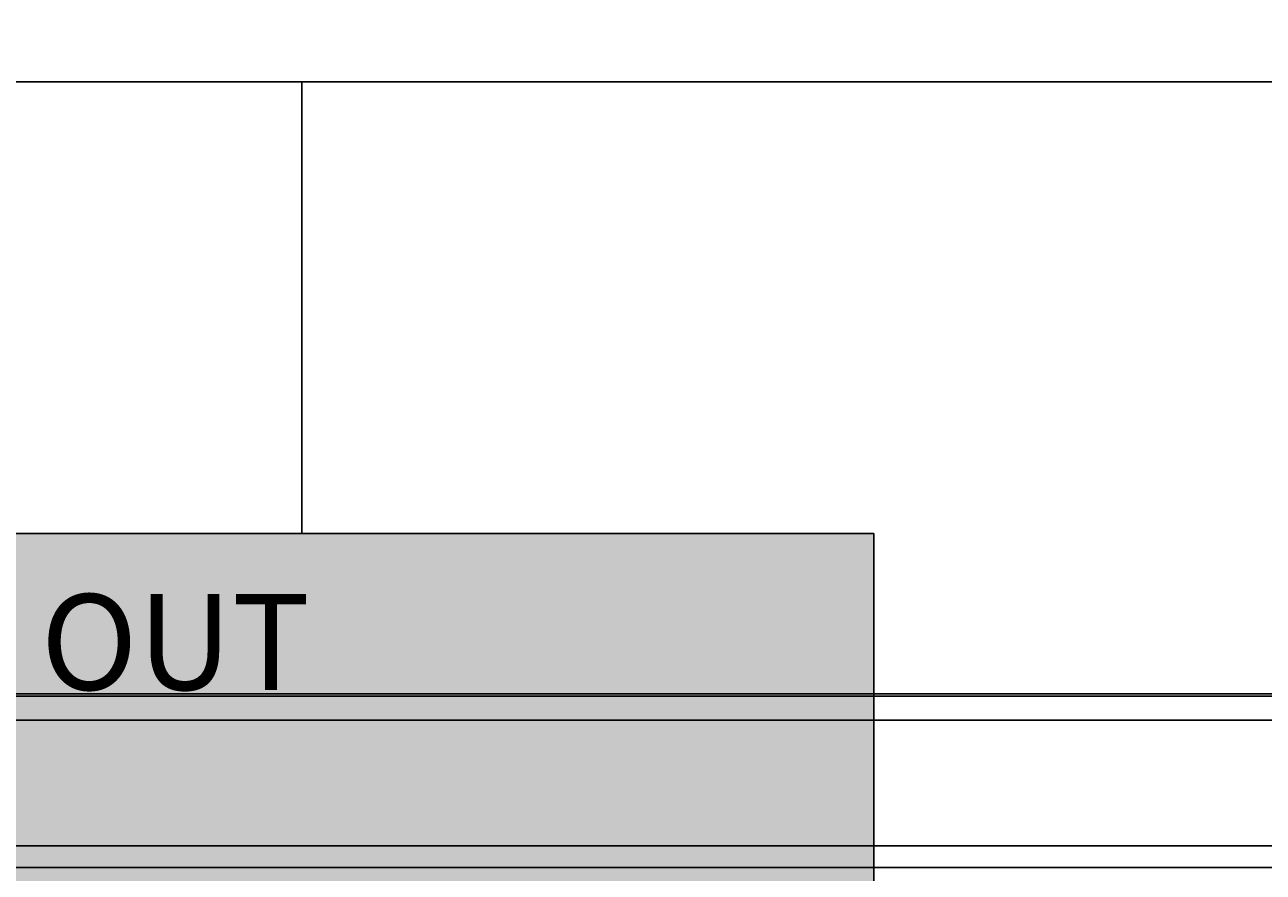
# Model space of a CAD drawing. Units: inches. Extents: x 35362 to 73946, y 43607 to 67532.
# Tile 6 of 134: x 37937 to 40793, y 48909 to 50863. Entities that reach past the tile are written whole.
import ezdxf

# ---------------------------------------------------------------- set-up
doc = ezdxf.new("R2010")
doc.units = ezdxf.units.IN
doc.header["$MEASUREMENT"] = 0
for name, color, linetype, lineweight in [('A-ANNO-DIMS', 2, 'Continuous', 18), ('E-ANNO-TEXT', 5, 'Continuous', 18), ('E-SYMB', 1, 'Continuous', 25), ('E-SYMB-PATT', 1, 'Continuous', 13), ('E-WIRE', 3, 'Continuous', 25)]:
    doc.layers.add(name, color=color, linetype=linetype, lineweight=lineweight)
doc.styles.get("Standard").update_dxf_attribs({"font": 'arial.ttf'})
doc.dimstyles.get("Standard").update_dxf_attribs({"dimtxt": 0.18, "dimasz": 0.18, "dimexe": 0.18, "dimexo": 0.0625, "dimgap": 0.09, "dimtad": 0, "dimtih": 1, "dimtoh": 1, "dimdec": 4, "dimzin": 0, "dimdsep": 46, "dimtxsty": 'Standard', "dimcen": 0.09, "dimadec": 0, "dimazin": 0, "dimtfac": 1, "dimtdec": 4, "dimtofl": 0, "dimtmove": 0, "dimatfit": 3, "dimfxl": 1, "dimtolj": 1, "dimtzin": 0, "dimarcsym": 0})

# ---------------------------------------------------------------- blocks, each defined once
blk = doc.blocks.new('*D40')
at = {"layer": 'A-ANNO-DIMS', "color": 0, "lineweight": -2, "transparency": 16777216}
for p, q in [((56873.5, 53351.5), (35361.8, 53351.5)), ((35361.9, 53351.3), (35361.9, 51333.3)), ((35361.9, 49314.8), (35361.9, 51332.9)), ((51806.5, 49314.7), (35361.8, 49314.7))]:
    blk.add_line(p, q, dxfattribs=at)
at = {"layer": 'A-ANNO-DIMS', "color": 0, "transparency": 16777216}
for points in [[(35361.9, 53351.3), (35362, 53351.3), (35361.9, 53351.5)], [(35361.9, 49314.8), (35362, 49314.8), (35361.9, 49314.7)]]:
    blk.add_solid(points, dxfattribs=at)
at = {"layer": 'Defpoints', "color": 0, "transparency": 16777216}
for p in [(35361.9, 53351.5), (56873.6, 53351.5), (51806.5, 49314.7)]:
    blk.add_point(p, dxfattribs=at)
at = {"layer": 'A-ANNO-DIMS', "color": 0, "transparency": 16777216, "insert": (35361.9, 51333.1), "char_height": 0.18, "attachment_point": 5}
blk.add_mtext('\\A1;4036.9', dxfattribs=at)
blk = doc.blocks.new('*D58')
at = {"layer": 'A-ANNO-DIMS', "color": 0, "lineweight": -2, "transparency": 16777216}
for p, q in [((38575.7, 50731.8), (35361.8, 50731.8)), ((35361.9, 50731.6), (35361.9, 50211)), ((35361.9, 49690), (35361.9, 50210.7)), ((38575.7, 49689.8), (35361.8, 49689.8))]:
    blk.add_line(p, q, dxfattribs=at)
at = {"layer": 'A-ANNO-DIMS', "color": 0, "transparency": 16777216}
for points in [[(35361.9, 50731.6), (35362, 50731.6), (35361.9, 50731.8)], [(35361.9, 49690), (35362, 49690), (35361.9, 49689.8)]]:
    blk.add_solid(points, dxfattribs=at)
at = {"layer": 'Defpoints', "color": 0, "transparency": 16777216}
for p in [(38575.8, 50731.8), (35361.9, 49689.8), (38575.8, 49689.8)]:
    blk.add_point(p, dxfattribs=at)
at = {"layer": 'A-ANNO-DIMS', "color": 0, "transparency": 16777216, "insert": (35361.9, 50210.8), "char_height": 0.18, "attachment_point": 5}
blk.add_mtext('\\A1;1042.0', dxfattribs=at)
blk = doc.blocks.new('*D67')
at = {"layer": 'A-ANNO-DIMS', "color": 0, "lineweight": -2, "transparency": 16777216}
for p, q in [((56873.5, 53351.5), (35361.8, 53351.5)), ((35361.9, 53351.3), (35361.9, 49400.9)), ((35361.9, 45450.1), (35361.9, 49400.5)), ((53793.6, 45449.9), (35361.8, 45449.9))]:
    blk.add_line(p, q, dxfattribs=at)
at = {"layer": 'A-ANNO-DIMS', "color": 0, "transparency": 16777216}
for points in [[(35361.9, 53351.3), (35362, 53351.3), (35361.9, 53351.5)], [(35361.9, 45450.1), (35362, 45450.1), (35361.9, 45449.9)]]:
    blk.add_solid(points, dxfattribs=at)
at = {"layer": 'Defpoints', "color": 0, "transparency": 16777216}
for p in [(35361.9, 53351.5), (56873.6, 53351.5), (53793.6, 45449.9)]:
    blk.add_point(p, dxfattribs=at)
at = {"layer": 'A-ANNO-DIMS', "color": 0, "transparency": 16777216, "insert": (35361.9, 49400.7), "char_height": 0.18, "attachment_point": 5}
blk.add_mtext('\\A1;7901.6', dxfattribs=at)
blk = doc.blocks.new('*D84')
at = {"layer": 'A-ANNO-DIMS', "color": 0, "lineweight": -2, "transparency": 16777216}
for p, q in [((55540.2, 49259.9), (35361.8, 49259.9)), ((35361.9, 49259.8), (35361.9, 49115.1)), ((35361.9, 48970.2), (35361.9, 49114.8)), ((55540.2, 48970), (35361.8, 48970))]:
    blk.add_line(p, q, dxfattribs=at)
at = {"layer": 'A-ANNO-DIMS', "color": 0, "transparency": 16777216}
for points in [[(35361.9, 49259.8), (35362, 49259.8), (35361.9, 49259.9)], [(35361.9, 48970.2), (35362, 48970.2), (35361.9, 48970)]]:
    blk.add_solid(points, dxfattribs=at)
at = {"layer": 'Defpoints', "color": 0, "transparency": 16777216}
for p in [(35361.9, 49259.9), (55540.3, 49259.9), (55540.3, 48970)]:
    blk.add_point(p, dxfattribs=at)
at = {"layer": 'A-ANNO-DIMS', "color": 0, "transparency": 16777216, "insert": (35361.9, 49115), "char_height": 0.18, "attachment_point": 5}
blk.add_mtext('\\A1;289.96', dxfattribs=at)
blk = doc.blocks.new('*D86')
at = {"layer": 'A-ANNO-DIMS', "color": 0, "lineweight": -2, "transparency": 16777216}
for p, q in [((51285.5, 49320.1), (35361.8, 49320.1)), ((35361.9, 49319.9), (35361.9, 49120.3)), ((35361.9, 48920.3), (35361.9, 49119.9)), ((51285.5, 48920.1), (35361.8, 48920.1))]:
    blk.add_line(p, q, dxfattribs=at)
at = {"layer": 'A-ANNO-DIMS', "color": 0, "transparency": 16777216}
for points in [[(35361.9, 49319.9), (35362, 49319.9), (35361.9, 49320.1)], [(35361.9, 48920.3), (35362, 48920.3), (35361.9, 48920.1)]]:
    blk.add_solid(points, dxfattribs=at)
at = {"layer": 'Defpoints', "color": 0, "transparency": 16777216}
for p in [(35361.9, 49320.1), (51285.6, 49320.1), (51285.6, 48920.1)]:
    blk.add_point(p, dxfattribs=at)
at = {"layer": 'A-ANNO-DIMS', "color": 0, "transparency": 16777216, "insert": (35361.9, 49120.1), "char_height": 0.18, "attachment_point": 5}
blk.add_mtext('\\A1;400.0', dxfattribs=at)

msp = doc.modelspace()

# ---------------------------------------------------------------- hatches: boundary and pattern name
at = {"layer": 'E-SYMB-PATT'}
h = msp.add_hatch(color=256, dxfattribs=at)
h.dxf.hatch_style = 1
h.paths.add_polyline_path([(39894.84, 49689.843), (37121.949, 49689.843), (37121.949, 46919.381), (39894.84, 46919.381)])

# ---------------------------------------------------------------- linework, layer by layer
at = {"layer": 'E-SYMB'}
msp.add_lwpolyline([(37121.949, 49689.843), (39894.84, 49689.843), (39894.84, 46919.381), (37121.949, 46919.381)], close=True, dxfattribs=at)
at = {"layer": 'E-WIRE'}
for p, q in [((38575.774, 49689.843), (38575.774, 50731.821)), ((38575.774, 50731.821), (54718.752, 50731.821))]:
    msp.add_line(p, q, dxfattribs=at)

# ---------------------------------------------------------------- texts
at = {"layer": 'E-ANNO-TEXT'}
msp.add_text('OUT', height=220.866, dxfattribs=at).set_placement((37974.012, 49329.39))

# ---------------------------------------------------------------- dimensions: what is measured, and where the dimension line sits
at = {"layer": 'A-ANNO-DIMS'}
for base, p1, p2, override, picture, middle in [((35361.949, 53351.529), (51806.517, 49314.669), (56873.602, 53351.529), {"dimdec": 1, "dimlfac": 1, "dimrnd": 0, "dimzin": 0, "dimdsep": 46, "dimlunit": 2}, '*D40', (35361.949, 51333.099)), ((35361.949, 53351.529), (53793.638, 45449.894), (56873.602, 53351.529), {"dimdec": 1, "dimlfac": 1, "dimrnd": 0, "dimzin": 0, "dimdsep": 46, "dimlunit": 2}, '*D67', (35361.949, 49400.712)), ((35361.949, 49689.843), (38575.774, 50731.821), (38575.774, 49689.843), {"dimdec": 1, "dimlfac": 1, "dimrnd": 0, "dimzin": 0, "dimdsep": 46, "dimlunit": 2}, '*D58', (35361.949, 50210.832)), ((35361.949, 49320.079), (51285.595, 48920.079), (51285.595, 49320.079), {"dimdec": 1, "dimlfac": 1, "dimrnd": 0, "dimzin": 0, "dimdsep": 46, "dimlunit": 2}, '*D86', (35361.949, 49120.079)), ((35361.9491, 49259.9353), (55540.2972, 48969.9796), (55540.2972, 49259.9353), {"dimdec": 2, "dimlfac": 1, "dimrnd": 0, "dimzin": 0, "dimdsep": 46, "dimlunit": 2}, '*D84', (35361.9491, 49114.9575))]:
    dim = msp.add_linear_dim(base=base, p1=p1, p2=p2, angle=90, dimstyle='Standard', override=override, dxfattribs=at)
    dim.commit()
    dim.dimension.update_dxf_attribs({"geometry": picture, "text_midpoint": middle})

doc.saveas('drawing.dxf')
